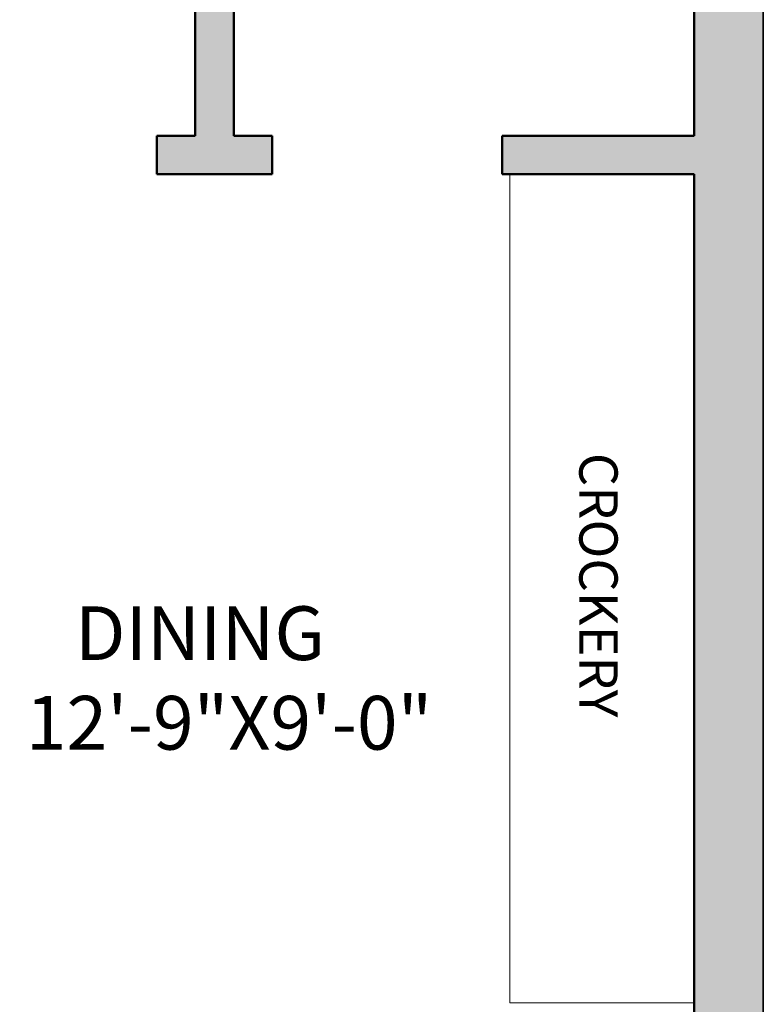
# Model space of a CAD drawing. Units: inches. Extents: x 1734 to 4011, y 1071 to 1891.
# Tile 22 of 27: x 3379 to 3476, y 1638 to 1766. Entities that reach past the tile are written whole.
import ezdxf

# ---------------------------------------------------------------- set-up
doc = ezdxf.new("R2010")
doc.units = ezdxf.units.IN
for name, color, linetype, lineweight in [('A-AREA-IDEN', 3, 'Continuous', 18), ('A-FURN', 8, 'Continuous', 18), ('A-WALL', 7, 'Continuous', 50), ('A-WALL-PATT', 8, 'Continuous', 13), ('C-PROP', 1, 'Continuous', 35)]:
    doc.layers.add(name, color=color, linetype=linetype, lineweight=lineweight)
doc.styles.get("Standard").update_dxf_attribs({"font": 'arial.ttf'})

msp = doc.modelspace()

# ---------------------------------------------------------------- hatches: boundary and pattern name
at = {"layer": 'A-WALL-PATT'}
h = msp.add_hatch(color=256, dxfattribs=at)
h.dxf.hatch_style = 1
h.paths.add_polyline_path([(3475.99, 1831.82), (3115.99, 1831.82), (3115.99, 1745.82), (3130.99, 1745.82), (3130.99, 1750.82), (3124.99, 1750.82), (3124.99, 1822.82), (3214.99, 1822.82), (3214.99, 1780.82), (3219.99, 1780.82), (3219.99, 1822.82), (3308.99, 1822.82), (3308.99, 1750.82), (3254.99, 1750.82), (3254.99, 1745.82), (3308.99, 1745.82), (3308.99, 1604.82), (3313.99, 1604.82), (3313.99, 1745.82), (3366.99, 1745.82), (3366.99, 1750.82), (3313.99, 1750.82), (3313.99, 1822.82), (3401.99, 1822.82), (3401.99, 1750.82), (3396.99, 1750.82), (3396.99, 1745.82), (3411.99, 1745.82), (3411.99, 1750.82), (3406.99, 1750.82), (3406.99, 1822.82), (3466.99, 1822.82), (3466.99, 1750.82), (3441.99, 1750.82), (3441.99, 1745.82), (3466.99, 1745.82), (3466.99, 1517.82), (3452.49, 1517.82), (3452.49, 1512.82), (3466.99, 1512.82), (3466.99, 1458.82), (3446.49, 1458.82), (3446.49, 1453.82), (3466.99, 1453.82), (3466.99, 1237.82), (3372.99, 1237.82), (3372.99, 1228.82), (3466.99, 1228.82), (3466.99, 1120.82), (3309.99, 1120.82), (3309.99, 1184.82), (3310.99, 1184.82), (3310.99, 1189.82), (3303.99, 1189.82), (3303.99, 1120.82), (3291.99, 1120.82), (3291.99, 1111.82), (3475.99, 1111.82)])
h.paths.add_polyline_path([(3169.99, 1745.82), (3224.99, 1745.82), (3224.99, 1750.82), (3154.99, 1750.82), (3154.99, 1745.82), (3160.99, 1745.82), (3160.99, 1636.82), (3169.99, 1636.82)], flags=17)
h.paths.add_polyline_path([(3169.99, 1588.82), (3160.99, 1588.82), (3160.99, 1559.82), (3313.99, 1559.82), (3313.99, 1568.82), (3308.99, 1568.82), (3308.99, 1564.82), (3169.99, 1564.82)], flags=17)
h.paths.add_polyline_path([(3416.49, 1517.82), (3401.99, 1517.82), (3401.99, 1512.82), (3416.49, 1512.82)], flags=17)
h.paths.add_polyline_path([(3371.99, 1517.82), (3366.99, 1517.82), (3366.99, 1453.82), (3392.49, 1453.82), (3392.49, 1458.82), (3371.99, 1458.82)], flags=17)
h.paths.add_polyline_path([(3258.99, 1529.82), (3160.99, 1529.82), (3160.99, 1494.82), (3169.99, 1494.82), (3169.99, 1524.82), (3253.99, 1524.82), (3253.99, 1520.82), (3258.99, 1520.82)], flags=17)
h.paths.add_polyline_path([(3263.99, 1458.82), (3258.99, 1458.82), (3258.99, 1490.82), (3253.99, 1490.82), (3253.99, 1458.82), (3169.99, 1458.82), (3169.99, 1470.82), (3160.99, 1470.82), (3160.99, 1387.82), (3169.99, 1387.82), (3169.99, 1453.82), (3263.99, 1453.82)], flags=17)
h.paths.add_polyline_path([(3313.99, 1453.82), (3318.99, 1453.82), (3318.99, 1458.82), (3299.99, 1458.82), (3299.99, 1453.82), (3308.99, 1453.82), (3308.99, 1321.82), (3266.49, 1321.82), (3266.49, 1312.82), (3313.99, 1312.82)], flags=17)
h.paths.add_polyline_path([(3212.49, 1321.82), (3169.99, 1321.82), (3169.99, 1339.82), (3160.99, 1339.82), (3160.99, 1312.82), (3212.49, 1312.82)], flags=17)
h.paths.add_polyline_path([(3313.99, 1288.82), (3304.99, 1288.82), (3304.99, 1285.82), (3313.99, 1285.82)], flags=17)
h.paths.add_polyline_path([(3324.99, 1237.82), (3304.99, 1237.82), (3304.99, 1228.82), (3324.99, 1228.82)], flags=17)

# ---------------------------------------------------------------- linework, layer by layer
at = {"layer": 'A-FURN'}
for p, q in [((3442.99, 1745.82), (3442.99, 1637.82)), ((3442.99, 1745.82), (3442.99, 1637.82)), ((3442.99, 1637.82), (3466.99, 1637.82))]:
    msp.add_line(p, q, dxfattribs=at)
at = {"layer": 'A-WALL'}
for p, q in [((3401.99, 1750.82), (3401.99, 1822.82)), ((3406.99, 1750.82), (3406.99, 1822.82)), ((3466.99, 1822.82), (3466.99, 1750.82)), ((3396.99, 1750.82), (3401.99, 1750.82)), ((3396.99, 1745.82), (3396.99, 1750.82)), ((3406.99, 1750.82), (3411.99, 1750.82)), ((3411.99, 1745.82), (3411.99, 1750.82)), ((3441.99, 1750.82), (3466.99, 1750.82)), ((3441.99, 1745.82), (3441.99, 1750.82)), ((3396.99, 1745.82), (3411.99, 1745.82)), ((3441.99, 1745.82), (3466.99, 1745.82)), ((3466.99, 1745.82), (3466.99, 1517.82))]:
    msp.add_line(p, q, dxfattribs=at)
at = {"layer": 'C-PROP'}
msp.add_lwpolyline([(3171.99, 1111.82), (3115.99, 1111.82), (3115.99, 1831.82), (3475.99, 1831.82), (3475.99, 1111.82), (3291.99, 1111.82)], dxfattribs=at)

# ---------------------------------------------------------------- texts
at = {"layer": 'A-AREA-IDEN', "insert": (3457.02, 1714.08), "char_height": 5, "attachment_point": 1, "rotation": 270}
msp.add_mtext_dynamic_manual_height_columns('   CROCKERY', width=86.9528, gutter_width=12.5, heights=[0], dxfattribs=at)
at = {"layer": 'A-AREA-IDEN', "insert": (3379.91, 1689.5), "char_height": 7, "attachment_point": 1}
msp.add_mtext_dynamic_manual_height_columns('   DINING\\P12\'-9"X9\'-0"', width=86.9528, gutter_width=12.5, heights=[0], dxfattribs=at)

doc.saveas('drawing.dxf')
